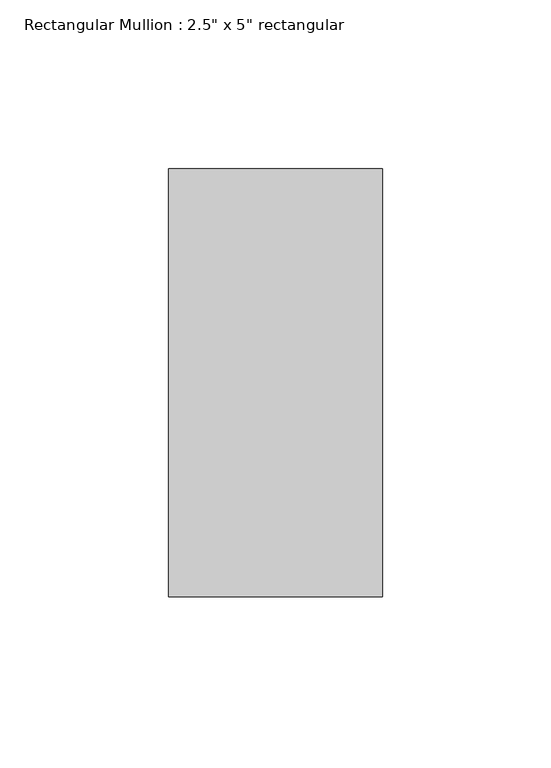
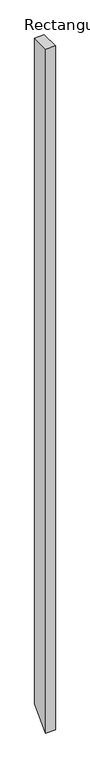
"""IFC4 building model written with IfcOpenShell, lengths in millimetres: member geometry."""

from ifc_helpers import new_model, si_unit, frame, origin, place, context, project, spatial, polyline, outline, extrude, source, transform, mapped, element, save


def member_aaec729c(model_context):
    return source(origin(), model_context, "Body", "SweptSolid", [
        extrude(outline(polyline([(-63.5, 0.0), (63.5, 0.0), (63.5, -4666.1970952), (-63.5, -4793.1970952), (-63.5, 0.0)])), frame((-63.5, 0.0, 0.0), z_axis=(1.0, 0.0, 0.0), x_axis=(0.0, 1.0, 0.0)), (0.0, 0.0, 1.0), 63.5),
    ])


if __name__ == "__main__":
    model = new_model("IFC4")
    model_context = context("Model", 3, world=origin())
    ifc_project = project(units=[si_unit("LENGTHUNIT", "METRE", prefix="MILLI")], contexts=[model_context])
    site = spatial("IfcSite", under=ifc_project)
    building = spatial("IfcBuilding", under=site)
    placement = place(None, origin())
    member_shape = member_aaec729c(model_context)
    element("IfcMember", 1, ObjectType="Rectangular Mullion : 2.5\" x 5\" rectangular", at=placement, inside=building, context=model_context, shape_type="MappedRepresentation", body=[
        mapped(member_shape, transform((0.0, 0.0, 0.0), x_axis=(1.0, 0.0, 0.0), y_axis=(0.0, 1.0, 0.0), z_axis=(0.0, 0.0, 1.0))),
    ])
    save(model, "model.ifc")

# Revit data of these elements
# Type "Rectangular Mullion : 2.5\" x 5\" rectangular"
#   built-in parameter 1007304 = 0.416667 (stored number, unit not read)
#   built-in parameter 1007301 = 0.104167 (stored number, unit not read)
#   built-in parameter 1007300 = 0.104167 (stored number, unit not read)
# Element 1 (IfcMember, "Rectangular Mullion : 2.5\" x 5\" rectangular")
#   Materials on its faces: "Aluminum"
# Materials
#   "Aluminum": class "Metal", colour RGB 247 247 247, transparency 0, Description = "Aluminum 6061", Cost = 0
